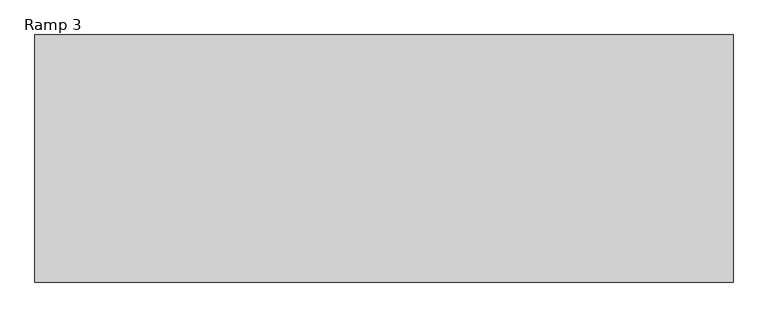
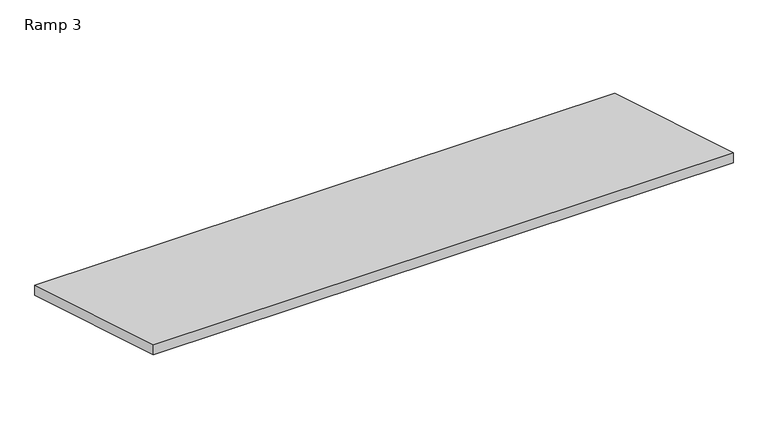
"""IFC4 building model written with IfcOpenShell, lengths in millimetres: ramp geometry, Ramp 3."""

from ifc_helpers import new_model, si_unit, frame, origin, place, context, project, spatial, polyline, outline, extrude, source, transform, mapped, element, save


def ramp_3_deb929ff(model_context):
    return source(origin(), model_context, "Body", "SweptSolid", [
        extrude(outline(polyline([(-5561.5027976, 457.2), (-4037.5027976, 0.0), (-4037.5027976, -79.5551356), (-5561.5027976, 377.6448644), (-5561.5027976, 457.2)])), frame((-19685.568705, 0.0, 0.0), z_axis=(1.0, 0.0, 0.0), x_axis=(0.0, 1.0, 0.0)), (0.0, 0.0, 1.0), 4305.3),
    ])


if __name__ == "__main__":
    model = new_model("IFC4")
    model_context = context("Model", 3, world=origin())
    ifc_project = project(units=[si_unit("LENGTHUNIT", "METRE", prefix="MILLI")], contexts=[model_context])
    site = spatial("IfcSite", under=ifc_project)
    building = spatial("IfcBuilding", under=site)
    placement = place(None, origin())
    ramp_3_shape = ramp_3_deb929ff(model_context)
    element("IfcRamp", 1, ObjectType="Ramp 3", at=placement, inside=building, context=model_context, shape_type="MappedRepresentation", body=[
        mapped(ramp_3_shape, transform((0.0, 0.0, 0.0), x_axis=(1.0, 0.0, 0.0), y_axis=(0.0, 1.0, 0.0), z_axis=(0.0, 0.0, 1.0))),
    ])
    save(model, "model.ifc")

# Revit data of these elements
# Element 1 (IfcRamp, "Ramp 3")
#   Materials on its faces: "Vinyl Composition Tile"
# Materials
#   "Vinyl Composition Tile": class "Generic", colour RGB 179 160 124, transparency 0, Description = "Vinyl Composition Tile", Cost = 0
